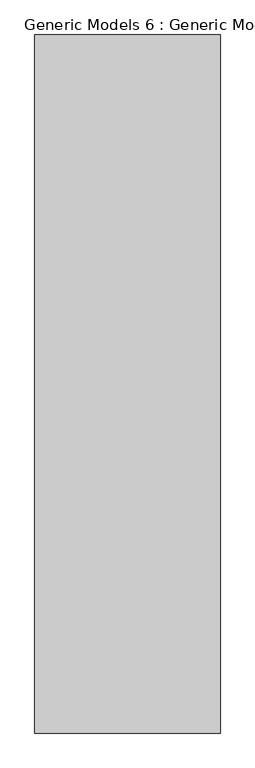
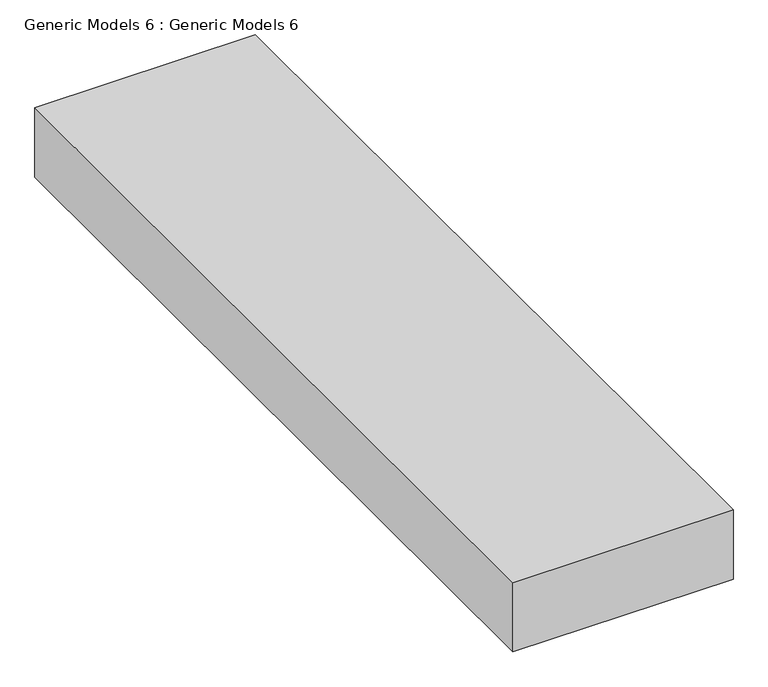
"""IFC4 building model written with IfcOpenShell, lengths in millimetres: proxy geometry, Generic Models 6 : Generic Models 6."""

from ifc_helpers import new_model, si_unit, frame, origin, place, context, project, spatial, polyline, outline, extrude, source, transform, mapped, element, save


def generic_models_6_generic_models_6_be8df775(model_context):
    return source(origin(), model_context, "Body", "SweptSolid", [
        extrude(outline(polyline([(-3344.0075703, -9934.1777232), (-3344.0075703, -11658.2905781), (-3802.4859258, -11658.2905781), (-3802.4859258, -9934.1777232), (-3344.0075703, -9934.1777232)])), frame((0.0, 0.0, 2520.0251482), z_axis=(0.0, 0.0, 1.0), x_axis=(1.0, 0.0, 0.0)), (0.0, 0.0, 1.0), 152.4),
    ])


if __name__ == "__main__":
    model = new_model("IFC4")
    model_context = context("Model", 3, world=origin())
    ifc_project = project(units=[si_unit("LENGTHUNIT", "METRE", prefix="MILLI")], contexts=[model_context])
    site = spatial("IfcSite", under=ifc_project)
    building = spatial("IfcBuilding", under=site)
    placement = place(None, origin())
    generic_models_6_generic_models_6_shape = generic_models_6_generic_models_6_be8df775(model_context)
    element("IfcBuildingElementProxy", 1, Name="Generic Models 6 : Generic Models 6", ObjectType="Generic Models 6 : Generic Models 6", at=placement, inside=building, context=model_context, shape_type="MappedRepresentation", body=[
        mapped(generic_models_6_generic_models_6_shape, transform((0.0, 0.0, 0.0), x_axis=(1.0, 0.0, 0.0), y_axis=(0.0, 1.0, 0.0), z_axis=(0.0, 0.0, 1.0))),
    ])
    save(model, "model.ifc")
